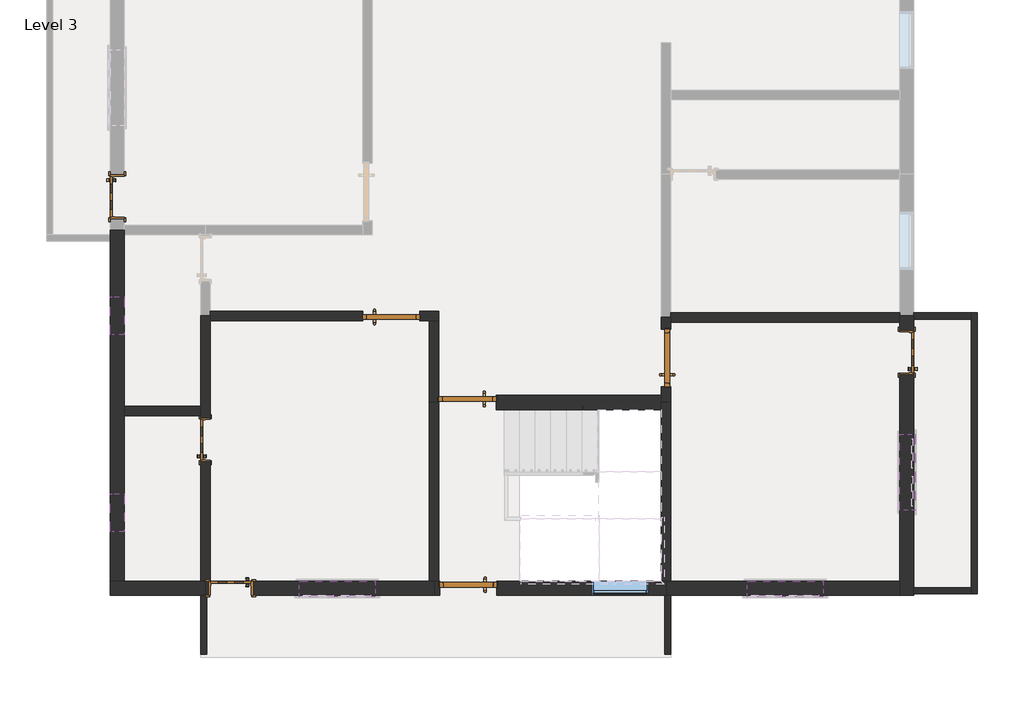
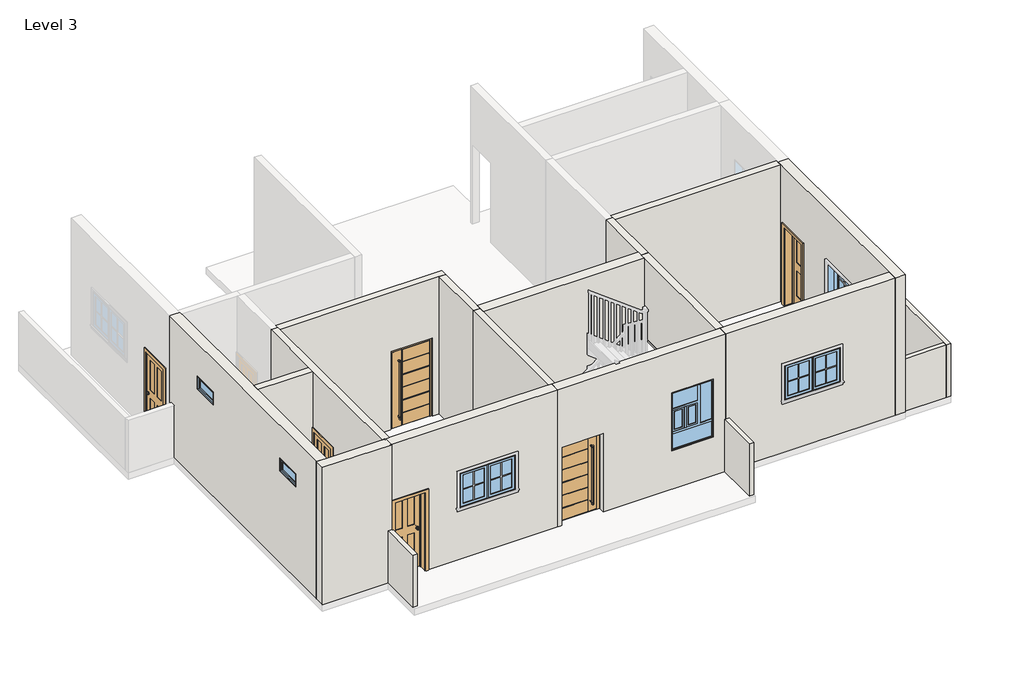
# One storey, part 1 of 3: 20 walls, 8 doors, 6 windows.
"""IFC4 building model written with IfcOpenShell, lengths in millimetres."""

from ifc_helpers import new_model, si_unit, frame, origin, place, context, project, spatial, polyline, outline, extrude, faceted_brep, transform, mapped, element, save
from components import door_3_44036f4b, door_3_3562bf2b, door_a03dd1d4, door_a34dad57, m_fixed_2_dd9f9b20, m_window_awning_double_horizontal_4_8afcb0b2, m_window_casement_double_sash_variable_3_661e274a

model = new_model("IFC4")

# Units and contexts
model_context = context("Model", 3, world=origin())
ifc_project = project(units=[si_unit("LENGTHUNIT", "METRE", prefix="MILLI")], contexts=[model_context])

# Site, building, storey
site = spatial("IfcSite", under=ifc_project)
building = spatial("IfcBuilding", under=site)
storey = spatial("IfcBuildingStorey", under=building, Name="Level 3", Elevation=6400.8)

# Doors
placement = place(None, origin())
door_3_shape = door_3_44036f4b(model_context)
element("IfcDoor", 1, ObjectType="3'", at=placement, inside=storey, context=model_context, shape_type="MappedRepresentation", body=[
    mapped(door_3_shape, transform((-13795.5794909, -9.3618509, 6400.8), x_axis=(1.0, 0.0, 0.0), y_axis=(0.0, 1.0, 0.0), z_axis=(0.0, 0.0, 1.0))),
])
element("IfcDoor", 2, ObjectType="3'", at=placement, inside=storey, context=model_context, shape_type="MappedRepresentation", body=[
    mapped(door_3_shape, transform((-9401.3794909, -682.4618509, 6400.8), x_axis=(0.0, 1.0, 0.0), y_axis=(-1.0, 0.0, 0.0), z_axis=(0.0, 0.0, 1.0))),
])
door_3_2_shape = door_3_3562bf2b(model_context)
element("IfcDoor", 3, ObjectType="3'", at=placement, inside=storey, context=model_context, shape_type="MappedRepresentation", body=[
    mapped(door_3_2_shape, transform((-12576.3794909, -1393.6618509, 6400.8), x_axis=(-1.0, 0.0, 0.0), y_axis=(0.0, -1.0, 0.0), z_axis=(0.0, 0.0, 1.0))),
])
element("IfcDoor", 4, ObjectType="3'", at=placement, inside=storey, context=model_context, shape_type="MappedRepresentation", body=[
    mapped(door_3_2_shape, transform((-12563.6794909, -4365.4618509, 6400.8), x_axis=(-1.0, 0.0, 0.0), y_axis=(0.0, -1.0, 0.0), z_axis=(0.0, 0.0, 1.0))),
])
door_shape = door_a03dd1d4(model_context)
element("IfcDoor", 5, ObjectType="M_Door-Interior-Single-4_Panel-Wood : 2'2\"", at=placement, inside=storey, context=model_context, shape_type="MappedRepresentation", body=[
    mapped(door_shape, transform((-16770.5544909, -1990.1618509, 6400.8), x_axis=(0.0, 1.0, 0.0), y_axis=(-1.0, 0.0, 0.0), z_axis=(0.0, 0.0, 1.0))),
])
door_2_shape = door_a34dad57(model_context)
element("IfcDoor", 6, ObjectType="M_Door-Interior-Single-4_Panel-Wood : 2'2\"", at=placement, inside=storey, context=model_context, shape_type="MappedRepresentation", body=[
    mapped(door_2_shape, transform((-18180.2544909, 1895.2381491, 6400.8), x_axis=(0.0, -1.0, 0.0), y_axis=(1.0, 0.0, 0.0), z_axis=(0.0, 0.0, 1.0))),
])
element("IfcDoor", 7, ObjectType="M_Door-Interior-Single-4_Panel-Wood : 2'2\"", at=placement, inside=storey, context=model_context, shape_type="MappedRepresentation", body=[
    mapped(door_2_shape, transform((-5550.1044909, -593.1618509, 6400.8), x_axis=(0.0, 1.0, 0.0), y_axis=(-1.0, 0.0, 0.0), z_axis=(0.0, 0.0, 1.0))),
])
element("IfcDoor", 8, ObjectType="M_Door-Interior-Single-4_Panel-Wood : 2'2\"", at=placement, inside=storey, context=model_context, shape_type="MappedRepresentation", body=[
    mapped(door_2_shape, transform((-16361.3794909, -4362.2868509, 6400.8), x_axis=(-1.0, 0.0, 0.0), y_axis=(0.0, -1.0, 0.0), z_axis=(0.0, 0.0, 1.0))),
])

# Walls
element("IfcWall", 9, ObjectType="Generic - 4\"", at=placement, inside=storey, context=model_context, shape_type="Brep", body=[
    faceted_brep([(-9325.1794909, -5419.5618509, 6400.8), (-9325.1794909, -4479.7618509, 6400.8), (-9325.1794909, -4479.7618509, 7620.0), (-9325.1794909, -5419.5618509, 7620.0), (-9426.7794909, -5419.5618509, 6400.8), (-9426.7794909, -5419.5618509, 7620.0), (-9426.7794909, -4479.7618509, 7620.0), (-9426.7794909, -4479.7618509, 6400.8), (-9401.3794909, -4479.7618509, 6400.8)], [[[0, 1, 2, 3]], [[4, 5, 6, 7]], [[1, 0, 4, 7, 8]], [[3, 2, 6, 5]], [[0, 3, 5, 4]], [[2, 1, 8, 7, 6]]]),
])
element("IfcWall", 10, ObjectType="Generic - 4\"", at=placement, inside=storey, context=model_context, shape_type="Brep", body=[
    faceted_brep([(-4422.9794909, -4454.3618509, 6400.8), (-4422.9794909, 41.4381491, 6400.8), (-4422.9794909, 41.4381491, 7620.0), (-4422.9794909, -4454.3618509, 7620.0), (-4524.5794909, -4454.3618509, 6400.8), (-4524.5794909, -4454.3618509, 7620.0), (-4524.5794909, -4352.7618509, 7620.0), (-4524.5794909, -60.1618509, 7620.0), (-4524.5794909, 41.4381491, 7620.0), (-4524.5794909, 41.4381491, 6400.8), (-4524.5794909, -60.1618509, 6400.8), (-4524.5794909, -4352.7618509, 6400.8)], [[[0, 1, 2, 3]], [[4, 5, 6, 7, 8, 9, 10, 11]], [[1, 0, 4, 11, 10, 9]], [[3, 2, 8, 7, 6, 5]], [[0, 3, 5, 4]], [[2, 1, 9, 8]]]),
])
element("IfcWall", 11, ObjectType="Generic - 4\"", at=placement, inside=storey, context=model_context, shape_type="SweptSolid", body=[
    extrude(outline(polyline([(-4524.5794909, -4454.3618509), (-5438.9794909, -4454.3618509), (-5438.9794909, -4352.7618509), (-4524.5794909, -4352.7618509), (-4524.5794909, -4454.3618509)])), frame((0.0, 0.0, 6400.8), z_axis=(0.0, 0.0, 1.0), x_axis=(1.0, 0.0, 0.0)), (0.0, 0.0, 1.0), 1219.2),
])
element("IfcWall", 12, ObjectType="Generic - 4\"", at=placement, inside=storey, context=model_context, shape_type="Brep", body=[
    faceted_brep([(-16843.5794909, -4479.7618509, 6400.8), (-16843.5794909, -5419.5618509, 6400.8), (-16843.5794909, -5419.5618509, 7620.0), (-16843.5794909, -4479.7618509, 7620.0), (-16741.9794909, -4479.7618509, 6400.8), (-16741.9794909, -4479.7618509, 7620.0), (-16741.9794909, -5419.5618509, 7620.0), (-16741.9794909, -5419.5618509, 6400.8), (-16792.7794909, -4479.7618509, 6400.8), (-16767.3794909, -4479.7618509, 6400.8)], [[[0, 1, 2, 3]], [[4, 5, 6, 7]], [[1, 0, 8, 9, 4, 7]], [[2, 1, 7, 6]], [[3, 2, 6, 5]], [[0, 3, 5, 4, 9, 8]]]),
])
element("IfcWall", 13, ObjectType="Generic - 4\"", at=placement, inside=storey, context=model_context, shape_type="Brep", body=[
    faceted_brep([(-4524.5794909, 41.4381491, 6400.8), (-5438.9794909, 41.4381491, 6400.8), (-5438.9794909, 41.4381491, 7620.0), (-4524.5794909, 41.4381491, 7620.0), (-4524.5794909, -60.1618509, 6400.8), (-4524.5794909, -60.1618509, 7620.0), (-5438.9794909, -60.1618509, 7620.0), (-5438.9794909, -60.1618509, 6400.8), (-5438.9794909, -34.7618509, 6400.8), (-5438.9794909, -9.3618509, 6400.8)], [[[0, 1, 2, 3]], [[4, 5, 6, 7]], [[1, 0, 4, 7, 8, 9]], [[3, 2, 6, 5]], [[0, 3, 5, 4]], [[2, 1, 9, 8, 7, 6]]]),
])
element("IfcWall", 14, ObjectType="Generic - 6\"", at=placement, inside=storey, context=model_context, shape_type="Brep", body=[
    faceted_brep([(-16691.1794909, -9.3618509, 6400.8), (-16691.1794909, -9.3618509, 9601.2), (-16691.1794909, -85.5618509, 9601.2), (-16691.1794909, -4251.1618509, 9601.2), (-16691.1794909, -4251.1618509, 6400.8), (-16691.1794909, -2345.3618509, 6400.8), (-16691.1794909, -2345.3618509, 8254.6), (-16691.1794909, -1634.9618509, 8254.6), (-16691.1794909, -1634.9618509, 6400.8), (-16691.1794909, -85.5618509, 6400.8), (-16843.5794909, -9.3618509, 9601.2), (-16843.5794909, -9.3618509, 6400.8), (-16843.5794909, -1457.1618509, 6400.8), (-16843.5794909, -1609.5618509, 6400.8), (-16843.5794909, -1634.9618509, 6400.8), (-16843.5794909, -1634.9618509, 8254.6), (-16843.5794909, -2345.3618509, 8254.6), (-16843.5794909, -2345.3618509, 6400.8), (-16843.5794909, -4251.1618509, 6400.8), (-16843.5794909, -4251.1618509, 9601.2), (-16843.5794909, -1609.5618509, 9601.2), (-16843.5794909, -1457.1618509, 9601.2), (-16716.5794909, -4251.1618509, 6400.8), (-16767.3794909, -4251.1618509, 6400.8), (-16792.7794909, -4251.1618509, 6400.8), (-16792.7794909, -4251.1618509, 9601.2), (-16767.3794909, -4251.1618509, 9601.2)], [[[0, 1, 2, 3, 4, 5, 6, 7, 8, 9]], [[10, 11, 12, 13, 14, 15, 16, 17, 18, 19, 20, 21]], [[4, 22, 23, 24, 18, 17, 5]], [[11, 0, 9, 8, 14, 13, 12]], [[1, 0, 11, 10]], [[3, 2, 1, 10, 21, 20, 19, 25, 26]], [[7, 15, 14, 8]], [[15, 7, 6, 16]], [[16, 6, 5, 17]], [[3, 26, 25, 19, 18, 24, 23, 22, 4]]]),
])
element("IfcWall", 15, ObjectType="Generic - 6\"", at=placement, inside=storey, context=model_context, shape_type="SweptSolid", body=[
    extrude(outline(polyline([(-16843.5794909, -1609.5618509), (-18062.7794909, -1609.5618509), (-18062.7794909, -1457.1618509), (-16843.5794909, -1457.1618509), (-16843.5794909, -1609.5618509)])), frame((0.0, 0.0, 6400.8), z_axis=(0.0, 0.0, 1.0), x_axis=(1.0, 0.0, 0.0)), (0.0, 0.0, 1.0), 3200.4),
])
element("IfcWall", 16, ObjectType="Generic - 6\"", at=placement, inside=storey, context=model_context, shape_type="Brep", body=[
    faceted_brep([(-13033.5794909, -85.5618509, 9601.2), (-13185.9794909, -85.5618509, 9601.2), (-16691.1794909, -85.5618509, 9601.2), (-16691.1794909, -85.5618509, 6400.8), (-14252.7794909, -85.5618509, 6400.8), (-14252.7794909, -85.5618509, 8229.6), (-13338.3794909, -85.5618509, 8229.6), (-13338.3794909, -85.5618509, 6400.8), (-13185.9794909, -85.5618509, 6400.8), (-13033.5794909, -85.5618509, 6400.8), (-16691.1794909, 66.8381491, 9601.2), (-13033.5794909, 66.8381491, 9601.2), (-13033.5794909, 66.8381491, 6400.8), (-13338.3794909, 66.8381491, 6400.8), (-13338.3794909, 66.8381491, 8229.6), (-14252.7794909, 66.8381491, 8229.6), (-14252.7794909, 66.8381491, 6400.8), (-16691.1794909, 66.8381491, 6400.8), (-13338.3794909, -65.5618509, 6400.8), (-13323.3794909, -65.5618509, 6400.8), (-13323.3794909, 11.4381491, 6400.8), (-13338.3794909, 11.4381491, 6400.8), (-16691.1794909, -9.3618509, 6400.8), (-14252.7794909, 11.4381491, 6400.8), (-14267.7794909, 11.4381491, 6400.8), (-14267.7794909, -65.5618509, 6400.8), (-14252.7794909, -65.5618509, 6400.8), (-16691.1794909, -9.3618509, 9601.2), (-14252.7794909, -65.5618509, 8229.6), (-13338.3794909, -65.5618509, 8229.6), (-13338.3794909, 11.4381491, 8229.6), (-14252.7794909, 11.4381491, 8229.6), (-14267.7794909, -65.5618509, 8244.6), (-14267.7794909, 11.4381491, 8244.6), (-13323.3794909, 11.4381491, 8244.6), (-13323.3794909, -65.5618509, 8244.6)], [[[0, 1, 2, 3, 4, 5, 6, 7, 8, 9]], [[10, 11, 12, 13, 14, 15, 16, 17]], [[12, 9, 8, 7, 18, 19, 20, 21, 13]], [[3, 22, 17, 16, 23, 24, 25, 26, 4]], [[2, 1, 0, 11, 10, 27]], [[3, 2, 27, 10, 17, 22]], [[0, 9, 12, 11]], [[5, 28, 29, 6]], [[14, 30, 31, 15]], [[6, 29, 18, 7]], [[30, 14, 13, 21]], [[28, 5, 4, 26]], [[15, 31, 23, 16]], [[32, 33, 34, 35]], [[35, 34, 20, 19]], [[31, 30, 21, 20, 34, 33, 24, 23]], [[33, 32, 25, 24]], [[29, 28, 26, 25, 32, 35, 19, 18]]]),
])
element("IfcWall", 17, ObjectType="Generic - 6\"", at=placement, inside=storey, context=model_context, shape_type="Brep", body=[
    faceted_brep([(-13185.9794909, -85.5618509, 6400.8), (-13185.9794909, -1393.6618509, 6400.8), (-13185.9794909, -1393.6618509, 9601.2), (-13185.9794909, -85.5618509, 9601.2), (-13033.5794909, -85.5618509, 9601.2), (-13033.5794909, -1279.3618509, 9601.2), (-13033.5794909, -1393.6618509, 9601.2), (-13033.5794909, -1393.6618509, 8229.6), (-13033.5794909, -1393.6618509, 6400.8), (-13033.5794909, -1376.3618508, 6400.8), (-13033.5794909, -1376.3618508, 8229.6), (-13033.5794909, -1376.3618508, 8244.6), (-13033.5794909, -1299.3618508, 8244.6), (-13033.5794909, -1299.3618508, 8229.6), (-13033.5794909, -1299.3618508, 6400.8), (-13033.5794909, -1279.3618508, 6400.8), (-13033.5794909, -85.5618509, 6400.8), (-13048.5794909, -1299.3618508, 6400.8), (-13048.5794909, -1376.3618508, 6400.8), (-13048.5794909, -1376.3618508, 8244.6), (-13048.5794909, -1299.3618508, 8244.6)], [[[0, 1, 2, 3]], [[4, 5, 6, 7, 8, 9, 10, 11, 12, 13, 14, 15, 16]], [[1, 0, 16, 15, 14, 17, 18, 9, 8]], [[2, 1, 8, 7, 6]], [[3, 2, 6, 5, 4]], [[0, 3, 4, 16]], [[19, 20, 12, 11]], [[20, 19, 18, 17]], [[18, 19, 11, 10, 9]], [[20, 17, 14, 13, 12]]]),
])
element("IfcWall", 18, ObjectType="Generic - 6\"", at=placement, inside=storey, context=model_context, shape_type="Brep", body=[
    faceted_brep([(-9325.1794909, -4251.1618509, 9601.2), (-9325.1794909, -4251.1618509, 6400.8), (-9325.1794909, -1393.6618509, 6400.8), (-9325.1794909, -1393.6618509, 9601.2), (-9477.5794909, -4251.1618509, 6400.8), (-9477.5794909, -4251.1618509, 9601.2), (-9477.5794909, -1507.9618509, 9601.2), (-9477.5794909, -1393.6618509, 9601.2), (-9477.5794909, -1393.6618509, 6400.8), (-9477.5794909, -1507.9618509, 6400.8), (-9401.3794909, -4251.1618509, 6400.8), (-9401.3794909, -4251.1618509, 9601.2)], [[[0, 1, 2, 3]], [[4, 5, 6, 7, 8, 9]], [[2, 1, 10, 4, 9, 8]], [[3, 2, 8, 7]], [[0, 3, 7, 6, 5, 11]], [[0, 11, 5, 4, 10, 1]]]),
])
element("IfcWall", 19, ObjectType="Generic - 6\"", at=placement, inside=storey, context=model_context, shape_type="Brep", body=[
    faceted_brep([(-5667.5794909, 41.4381491, 9601.2), (-5667.5794909, 41.4381491, 6400.8), (-9325.1794909, 41.4381491, 6400.8), (-9325.1794909, 41.4381491, 9601.2), (-5667.5794909, -110.9618509, 6400.8), (-5667.5794909, -110.9618509, 9601.2), (-9325.1794909, -110.9618509, 9601.2), (-9325.1794909, -110.9618509, 6400.8), (-5667.5794909, -9.3618509, 6400.8), (-5667.5794909, -34.7618509, 6400.8), (-9325.1794909, -34.7618509, 6400.8), (-9325.1794909, -34.7618509, 9601.2), (-5667.5794909, -34.7618509, 9601.2), (-5667.5794909, -9.3618509, 9601.2)], [[[0, 1, 2, 3]], [[4, 5, 6, 7]], [[2, 1, 8, 9, 4, 7, 10]], [[0, 3, 11, 6, 5, 12, 13]], [[3, 2, 10, 7, 6, 11]], [[0, 13, 12, 5, 4, 9, 8, 1]]]),
])
element("IfcWall", 20, ObjectType="Generic - 6\"", at=placement, inside=storey, context=model_context, shape_type="Brep", body=[
    faceted_brep([(-9325.1794909, -34.7618509, 6400.8), (-9325.1794909, -34.7618509, 9601.2), (-9325.1794909, -110.9618509, 9601.2), (-9325.1794909, -1393.6618509, 9601.2), (-9325.1794909, -1393.6618509, 6400.8), (-9325.1794909, -1139.6618509, 6400.8), (-9325.1794909, -1139.6618509, 8229.6), (-9325.1794909, -225.2618509, 8229.6), (-9325.1794909, -225.2618509, 6400.8), (-9325.1794909, -110.9618509, 6400.8), (-9477.5794909, -34.7618509, 9601.2), (-9477.5794909, -34.7618509, 6400.8), (-9477.5794909, -225.2618509, 6400.8), (-9477.5794909, -225.2618509, 8229.6), (-9477.5794909, -1139.6618509, 8229.6), (-9477.5794909, -1139.6618509, 6400.8), (-9477.5794909, -1279.3618509, 6400.8), (-9477.5794909, -1393.6618509, 6400.8), (-9477.5794909, -1393.6618509, 9601.2), (-9477.5794909, -1279.3618509, 9601.2), (-9345.1794909, -225.2618509, 6400.8), (-9345.1794909, -210.2618509, 6400.8), (-9422.1794909, -210.2618509, 6400.8), (-9422.1794909, -225.2618509, 6400.8), (-9422.1794909, -1139.6618509, 6400.8), (-9422.1794909, -1154.6618509, 6400.8), (-9345.1794909, -1154.6618509, 6400.8), (-9345.1794909, -1139.6618509, 6400.8), (-9345.1794909, -1139.6618509, 8229.6), (-9345.1794909, -225.2618509, 8229.6), (-9422.1794909, -225.2618509, 8229.6), (-9422.1794909, -1139.6618509, 8229.6), (-9345.1794909, -1154.6618509, 8244.6), (-9422.1794909, -1154.6618509, 8244.6), (-9422.1794909, -210.2618509, 8244.6), (-9345.1794909, -210.2618509, 8244.6)], [[[0, 1, 2, 3, 4, 5, 6, 7, 8, 9]], [[10, 11, 12, 13, 14, 15, 16, 17, 18, 19]], [[11, 0, 9, 8, 20, 21, 22, 23, 12]], [[4, 17, 16, 15, 24, 25, 26, 27, 5]], [[1, 0, 11, 10]], [[3, 2, 1, 10, 19, 18]], [[4, 3, 18, 17]], [[6, 28, 29, 7]], [[13, 30, 31, 14]], [[30, 13, 12, 23]], [[7, 29, 20, 8]], [[14, 31, 24, 15]], [[28, 6, 5, 27]], [[32, 33, 34, 35]], [[35, 34, 22, 21]], [[31, 30, 23, 22, 34, 33, 25, 24]], [[33, 32, 26, 25]], [[29, 28, 27, 26, 32, 35, 21, 20]]]),
])
element("IfcWall", 21, ObjectType="Generic - 6\"", at=placement, inside=storey, context=model_context, shape_type="Brep", body=[
    faceted_brep([(-13185.9794909, -1393.6618509, 6400.8), (-13185.9794909, -4251.1618509, 6400.8), (-13185.9794909, -4251.1618509, 9601.2), (-13185.9794909, -1393.6618509, 9601.2), (-13033.5794909, -1393.6618509, 9601.2), (-13033.5794909, -1507.9618509, 9601.2), (-13033.5794909, -4251.1618509, 9601.2), (-13033.5794909, -4251.1618509, 6400.8), (-13033.5794909, -1507.9618509, 6400.8), (-13033.5794909, -1393.6618509, 6400.8), (-13033.5794909, -1393.6618509, 8229.6), (-13109.7794909, -4251.1618509, 6400.8), (-13109.7794909, -4251.1618509, 9601.2)], [[[0, 1, 2, 3]], [[4, 5, 6, 7, 8, 9, 10]], [[1, 0, 9, 8, 7, 11]], [[3, 2, 12, 6, 5, 4]], [[0, 3, 4, 10, 9]], [[2, 1, 11, 7, 6, 12]]]),
])
element("IfcWall", 22, ObjectType="Generic - 9\"", at=placement, inside=storey, context=model_context, shape_type="Brep", body=[
    faceted_brep([(-5667.5794909, -4251.1618509, 9601.2), (-5667.5794909, -4251.1618509, 6400.8), (-9325.1794909, -4251.1618509, 6400.8), (-9401.3794909, -4251.1618509, 6400.8), (-9401.3794909, -4251.1618509, 9601.2), (-9325.1794909, -4251.1618509, 9601.2), (-8105.9794909, -4251.1618509, 8420.0), (-8105.9794909, -4251.1618509, 7620.0), (-6886.7794909, -4251.1618509, 7620.0), (-6886.7794909, -4251.1618509, 8420.0), (-5667.5794909, -4479.7618509, 6400.8), (-5667.5794909, -4479.7618509, 9601.2), (-9401.3794909, -4479.7618509, 9601.2), (-9401.3794909, -4479.7618509, 6400.8), (-9325.1794909, -4479.7618509, 6400.8), (-8105.9794909, -4479.7618509, 8420.0), (-6886.7794909, -4479.7618509, 8420.0), (-6886.7794909, -4479.7618509, 7620.0), (-8105.9794909, -4479.7618509, 7620.0)], [[[0, 1, 2, 3, 4, 5], [6, 7, 8, 9]], [[10, 11, 12, 13, 14], [15, 16, 17, 18]], [[3, 2, 1, 10, 14, 13]], [[4, 3, 13, 12]], [[0, 5, 4, 12, 11]], [[0, 11, 10, 1]], [[7, 6, 15, 18]], [[8, 7, 18, 17]], [[9, 8, 17, 16]], [[6, 9, 16, 15]]]),
])
element("IfcWall", 23, ObjectType="Generic - 9\"", at=placement, inside=storey, context=model_context, shape_type="Brep", body=[
    faceted_brep([(-18062.7794909, -4251.1618509, 6400.8), (-18062.7794909, -1609.5618509, 6400.8), (-18062.7794909, -1457.1618509, 6400.8), (-18062.7794909, 1286.0381491, 6400.8), (-18062.7794909, 1362.2381491, 6400.8), (-18062.7794909, 1362.2381491, 9601.2), (-18062.7794909, 1286.0381491, 9601.2), (-18062.7794909, -1457.1618509, 9601.2), (-18062.7794909, -1609.5618509, 9601.2), (-18062.7794909, -4251.1618509, 9601.2), (-18062.7794909, -3463.7618509, 8534.4), (-18062.7794909, -3463.7618509, 8839.2), (-18062.7794909, -2854.1618509, 8839.2), (-18062.7794909, -2854.1618509, 8534.4), (-18062.7794909, -314.1618509, 8534.4), (-18062.7794909, -314.1618509, 8839.2), (-18062.7794909, 295.4381491, 8839.2), (-18062.7794909, 295.4381491, 8534.4), (-18291.3794909, -4251.1618509, 6400.8), (-18291.3794909, -4251.1618509, 9601.2), (-18291.3794909, 1362.2381491, 9601.2), (-18291.3794909, 1362.2381491, 6400.8), (-18291.3794909, 1286.0381491, 6400.8), (-18291.3794909, 1184.4381491, 6400.8), (-18291.3794909, -3463.7618509, 8534.4), (-18291.3794909, -2854.1618509, 8534.4), (-18291.3794909, -2854.1618509, 8839.2), (-18291.3794909, -3463.7618509, 8839.2), (-18291.3794909, -314.1618509, 8534.4), (-18291.3794909, 295.4381491, 8534.4), (-18291.3794909, 295.4381491, 8839.2), (-18291.3794909, -314.1618509, 8839.2)], [[[0, 1, 2, 3, 4, 5, 6, 7, 8, 9], [10, 11, 12, 13], [14, 15, 16, 17]], [[18, 19, 20, 21, 22, 23], [24, 25, 26, 27], [28, 29, 30, 31]], [[4, 3, 2, 1, 0, 18, 23, 22, 21]], [[9, 8, 7, 6, 5, 20, 19]], [[0, 9, 19, 18]], [[11, 10, 24, 27]], [[12, 11, 27, 26]], [[13, 12, 26, 25]], [[10, 13, 25, 24]], [[15, 14, 28, 31]], [[16, 15, 31, 30]], [[17, 16, 30, 29]], [[14, 17, 29, 28]], [[4, 21, 20, 5]]]),
])
element("IfcWall", 24, ObjectType="Generic - 9\"", at=placement, inside=storey, context=model_context, shape_type="Brep", body=[
    faceted_brep([(-13033.5794909, -1279.3618509, 9601.2), (-9477.5794909, -1279.3618509, 9601.2), (-9477.5794909, -1279.3618509, 6400.8), (-12119.1794909, -1279.3618509, 6400.8), (-12119.1794909, -1279.3618509, 8229.6), (-13033.5794909, -1279.3618509, 8229.6), (-9477.5794909, -1507.9618509, 9601.2), (-13033.5794909, -1507.9618509, 9601.2), (-13033.5794909, -1507.9618509, 8229.6), (-12119.1794909, -1507.9618509, 8229.6), (-12119.1794909, -1507.9618509, 6400.8), (-9477.5794909, -1507.9618509, 6400.8), (-9477.5794909, -1393.6618509, 6400.8), (-12119.1794909, -1376.3618508, 6400.8), (-12104.1794909, -1376.3618508, 6400.8), (-12104.1794909, -1299.3618508, 6400.8), (-12119.1794909, -1299.3618508, 6400.8), (-13033.5794909, -1393.6618509, 9601.2), (-9477.5794909, -1393.6618509, 9601.2), (-13033.5794909, -1299.3618508, 8229.6), (-13033.5794909, -1299.3618508, 8244.6), (-13033.5794909, -1376.3618508, 8244.6), (-13033.5794909, -1376.3618508, 8229.6), (-12119.1794909, -1299.3618508, 8229.6), (-12119.1794909, -1376.3618508, 8229.6), (-12104.1794909, -1299.3618508, 8244.6), (-12104.1794909, -1376.3618508, 8244.6)], [[[0, 1, 2, 3, 4, 5]], [[6, 7, 8, 9, 10, 11]], [[2, 12, 11, 10, 13, 14, 15, 16, 3]], [[1, 0, 17, 7, 6, 18]], [[7, 17, 0, 5, 19, 20, 21, 22, 8]], [[2, 1, 18, 6, 11, 12]], [[4, 23, 19, 5]], [[22, 24, 9, 8]], [[23, 4, 3, 16]], [[9, 24, 13, 10]], [[25, 26, 21, 20]], [[24, 22, 21, 26, 14, 13]], [[26, 25, 15, 14]], [[19, 23, 16, 15, 25, 20]]]),
])
element("IfcWall", 25, ObjectType="Generic - 9\"", at=placement, inside=storey, context=model_context, shape_type="Brep", body=[
    faceted_brep([(-5667.5794909, -4479.7618509, 9601.2), (-5667.5794909, -4251.1618509, 9601.2), (-5667.5794909, -110.9618509, 9601.2), (-5667.5794909, -9.3618509, 9601.2), (-5667.5794909, -9.3618509, 6400.8), (-5667.5794909, -110.9618509, 6400.8), (-5667.5794909, -237.9618509, 6400.8), (-5667.5794909, -237.9618509, 8254.6), (-5667.5794909, -948.3618509, 8254.6), (-5667.5794909, -948.3618509, 6400.8), (-5667.5794909, -4251.1618509, 6400.8), (-5667.5794909, -4479.7618509, 6400.8), (-5667.5794909, -3120.0618509, 8420.0), (-5667.5794909, -3120.0618509, 7620.0), (-5667.5794909, -1900.8618509, 7620.0), (-5667.5794909, -1900.8618509, 8420.0), (-5438.9794909, -9.3618509, 9601.2), (-5438.9794909, -4479.7618509, 9601.2), (-5438.9794909, -4479.7618509, 6400.8), (-5438.9794909, -4454.3618509, 6400.8), (-5438.9794909, -4352.7618509, 6400.8), (-5438.9794909, -948.3618509, 6400.8), (-5438.9794909, -948.3618509, 8254.6), (-5438.9794909, -237.9618509, 8254.6), (-5438.9794909, -237.9618509, 6400.8), (-5438.9794909, -60.1618509, 6400.8), (-5438.9794909, -9.3618509, 6400.8), (-5438.9794909, -3120.0618509, 8420.0), (-5438.9794909, -1900.8618509, 8420.0), (-5438.9794909, -1900.8618509, 7620.0), (-5438.9794909, -3120.0618509, 7620.0)], [[[0, 1, 2, 3, 4, 5, 6, 7, 8, 9, 10, 11], [12, 13, 14, 15]], [[16, 17, 18, 19, 20, 21, 22, 23, 24, 25, 26], [27, 28, 29, 30]], [[4, 26, 25, 24, 6, 5]], [[18, 11, 10, 9, 21, 20, 19]], [[3, 2, 1, 0, 17, 16]], [[11, 18, 17, 0]], [[12, 15, 28, 27]], [[15, 14, 29, 28]], [[14, 13, 30, 29]], [[13, 12, 27, 30]], [[3, 16, 26, 4]], [[23, 7, 6, 24]], [[7, 23, 22, 8]], [[8, 22, 21, 9]]]),
])
element("IfcWall", 26, ObjectType="Generic - 9\"", at=placement, inside=storey, context=model_context, shape_type="Brep", body=[
    faceted_brep([(-13109.7794909, -4251.1618509, 6400.8), (-13109.7794909, -4251.1618509, 9601.2), (-13033.5794909, -4251.1618509, 9601.2), (-9477.5794909, -4251.1618509, 9601.2), (-9401.3794909, -4251.1618509, 9601.2), (-9401.3794909, -4251.1618509, 6400.8), (-9477.5794909, -4251.1618509, 6400.8), (-12106.4794909, -4251.1618509, 6400.8), (-12106.4794909, -4251.1618509, 8229.6), (-13020.8794909, -4251.1618509, 8229.6), (-13020.8794909, -4251.1618509, 6400.8), (-13033.5794909, -4251.1618509, 6400.8), (-10595.1794909, -4251.1618509, 8650.8), (-10595.1794909, -4251.1618509, 7300.8), (-9680.7794909, -4251.1618509, 7300.8), (-9680.7794909, -4251.1618509, 8650.8), (-13109.7794909, -4479.7618509, 9601.2), (-13109.7794909, -4479.7618509, 6400.8), (-13020.8794909, -4479.7618509, 6400.8), (-13020.8794909, -4479.7618509, 8229.6), (-12106.4794909, -4479.7618509, 8229.6), (-12106.4794909, -4479.7618509, 6400.8), (-9426.7794909, -4479.7618509, 6400.8), (-9401.3794909, -4479.7618509, 6400.8), (-9401.3794909, -4479.7618509, 9601.2), (-10595.1794909, -4479.7618509, 8650.8), (-9680.7794909, -4479.7618509, 8650.8), (-9680.7794909, -4479.7618509, 7300.8), (-10595.1794909, -4479.7618509, 7300.8), (-12106.4794909, -4348.1618508, 6400.8), (-12091.4794909, -4348.1618508, 6400.8), (-12091.4794909, -4271.1618508, 6400.8), (-12106.4794909, -4271.1618508, 6400.8), (-13020.8794909, -4271.1618508, 6400.8), (-13035.8794909, -4271.1618508, 6400.8), (-13035.8794909, -4348.1618508, 6400.8), (-13020.8794909, -4348.1618508, 6400.8), (-12106.4794909, -4271.1618508, 8229.6), (-13020.8794909, -4271.1618508, 8229.6), (-13020.8794909, -4348.1618508, 8229.6), (-12106.4794909, -4348.1618508, 8229.6), (-12091.4794909, -4271.1618508, 8244.6), (-12091.4794909, -4348.1618508, 8244.6), (-13035.8794909, -4348.1618508, 8244.6), (-13035.8794909, -4271.1618508, 8244.6)], [[[0, 1, 2, 3, 4, 5, 6, 7, 8, 9, 10, 11], [12, 13, 14, 15]], [[16, 17, 18, 19, 20, 21, 22, 23, 24], [25, 26, 27, 28]], [[5, 23, 22, 21, 29, 30, 31, 32, 7, 6]], [[17, 0, 11, 10, 33, 34, 35, 36, 18]], [[1, 0, 17, 16]], [[4, 3, 2, 1, 16, 24]], [[8, 37, 38, 9]], [[19, 39, 40, 20]], [[39, 19, 18, 36]], [[9, 38, 33, 10]], [[20, 40, 29, 21]], [[37, 8, 7, 32]], [[41, 42, 43, 44]], [[44, 43, 35, 34]], [[40, 39, 36, 35, 43, 42, 30, 29]], [[42, 41, 31, 30]], [[38, 37, 32, 31, 41, 44, 34, 33]], [[12, 15, 26, 25]], [[15, 14, 27, 26]], [[14, 13, 28, 27]], [[13, 12, 25, 28]], [[4, 24, 23, 5]]]),
])
element("IfcWall", 27, ObjectType="Generic - 9\"", at=placement, inside=storey, context=model_context, shape_type="Brep", body=[
    faceted_brep([(-16792.7794909, -4251.1618509, 9601.2), (-16691.1794909, -4251.1618509, 9601.2), (-13185.9794909, -4251.1618509, 9601.2), (-13109.7794909, -4251.1618509, 9601.2), (-13109.7794909, -4251.1618509, 6400.8), (-13185.9794909, -4251.1618509, 6400.8), (-16006.1794909, -4251.1618509, 6400.8), (-16006.1794909, -4251.1618509, 8254.6), (-16716.5794909, -4251.1618509, 8254.6), (-16716.5794909, -4251.1618509, 6400.8), (-16792.7794909, -4251.1618509, 6400.8), (-15269.5794909, -4251.1618509, 8420.0), (-15269.5794909, -4251.1618509, 7620.0), (-14050.3794909, -4251.1618509, 7620.0), (-14050.3794909, -4251.1618509, 8420.0), (-13109.7794909, -4479.7618509, 9601.2), (-16792.7794909, -4479.7618509, 9601.2), (-16792.7794909, -4479.7618509, 6400.8), (-16741.9794909, -4479.7618509, 6400.8), (-16716.5794909, -4479.7618509, 6400.8), (-16716.5794909, -4479.7618509, 8254.6), (-16006.1794909, -4479.7618509, 8254.6), (-16006.1794909, -4479.7618509, 6400.8), (-13109.7794909, -4479.7618509, 6400.8), (-15269.5794909, -4479.7618509, 8420.0), (-14050.3794909, -4479.7618509, 8420.0), (-14050.3794909, -4479.7618509, 7620.0), (-15269.5794909, -4479.7618509, 7620.0)], [[[0, 1, 2, 3, 4, 5, 6, 7, 8, 9, 10], [11, 12, 13, 14]], [[15, 16, 17, 18, 19, 20, 21, 22, 23], [24, 25, 26, 27]], [[17, 10, 9, 19, 18]], [[4, 23, 22, 6, 5]], [[3, 2, 1, 0, 16, 15]], [[4, 3, 15, 23]], [[11, 14, 25, 24]], [[14, 13, 26, 25]], [[13, 12, 27, 26]], [[12, 11, 24, 27]], [[8, 20, 19, 9]], [[20, 8, 7, 21]], [[21, 7, 6, 22]], [[10, 17, 16, 0]]]),
])
element("IfcWall", 28, ObjectType="Generic - 9\"", at=placement, inside=storey, context=model_context, shape_type="Brep", body=[
    faceted_brep([(-16767.3794909, -4251.1618509, 9601.2), (-16767.3794909, -4251.1618509, 6400.8), (-16843.5794909, -4251.1618509, 6400.8), (-18062.7794909, -4251.1618509, 6400.8), (-18291.3794909, -4251.1618509, 6400.8), (-18291.3794909, -4251.1618509, 9601.2), (-18062.7794909, -4251.1618509, 9601.2), (-16843.5794909, -4251.1618509, 9601.2), (-16767.3794909, -4479.7618509, 6400.8), (-16767.3794909, -4479.7618509, 9601.2), (-18291.3794909, -4479.7618509, 9601.2), (-18291.3794909, -4479.7618509, 6400.8), (-16843.5794909, -4479.7618509, 6400.8)], [[[0, 1, 2, 3, 4, 5, 6, 7]], [[8, 9, 10, 11, 12]], [[4, 3, 2, 1, 8, 12, 11]], [[0, 7, 6, 5, 10, 9]], [[5, 4, 11, 10]], [[0, 9, 8, 1]]]),
])

# Windows
m_fixed_2_shape = m_fixed_2_dd9f9b20(model_context)
element("IfcWindow", 29, ObjectType="M_Fixed : 2'", at=placement, inside=storey, context=model_context, shape_type="MappedRepresentation", body=[
    mapped(m_fixed_2_shape, transform((-18164.0794909, -3158.9618509, 7619.4), x_axis=(0.0, 1.0, 0.0), y_axis=(-1.0, 0.0, 0.0), z_axis=(0.0, 0.0, 1.0))),
])
element("IfcWindow", 30, ObjectType="M_Fixed : 2'", at=placement, inside=storey, context=model_context, shape_type="MappedRepresentation", body=[
    mapped(m_fixed_2_shape, transform((-18164.0794909, -9.3618509, 7619.4), x_axis=(0.0, 1.0, 0.0), y_axis=(-1.0, 0.0, 0.0), z_axis=(0.0, 0.0, 1.0))),
])
m_window_awning_double_horizontal_4_shape = m_window_awning_double_horizontal_4_8afcb0b2(model_context)
element("IfcWindow", 31, ObjectType="M_Window-Awning-Double-Horizontal : 4'", at=placement, inside=storey, context=model_context, shape_type="MappedRepresentation", body=[
    mapped(m_window_awning_double_horizontal_4_shape, transform((-14659.9794909, -4365.4618509, 6720.0), x_axis=(-1.0, 0.0, 0.0), y_axis=(0.0, -1.0, 0.0), z_axis=(0.0, 0.0, 1.0))),
])
element("IfcWindow", 32, ObjectType="M_Window-Awning-Double-Horizontal : 4'", at=placement, inside=storey, context=model_context, shape_type="MappedRepresentation", body=[
    mapped(m_window_awning_double_horizontal_4_shape, transform((-5553.2794909, -2510.4618509, 6720.0), x_axis=(0.0, -1.0, 0.0), y_axis=(1.0, 0.0, 0.0), z_axis=(0.0, 0.0, 1.0))),
])
element("IfcWindow", 33, ObjectType="M_Window-Awning-Double-Horizontal : 4'", at=placement, inside=storey, context=model_context, shape_type="MappedRepresentation", body=[
    mapped(m_window_awning_double_horizontal_4_shape, transform((-7496.3794909, -4365.4618509, 6720.0), x_axis=(-1.0, 0.0, 0.0), y_axis=(0.0, -1.0, 0.0), z_axis=(0.0, 0.0, 1.0))),
])
m_window_casement_double_sash_variable_3_shape = m_window_casement_double_sash_variable_3_661e274a(model_context)
element("IfcWindow", 34, ObjectType="M_Window-Casement-Double-Sash-Variable : 3'", at=placement, inside=storey, context=model_context, shape_type="MappedRepresentation", body=[
    mapped(m_window_casement_double_sash_variable_3_shape, transform((-10137.9794909, -4365.4618509, 6400.8), x_axis=(-1.0, 0.0, 0.0), y_axis=(0.0, -1.0, 0.0), z_axis=(0.0, 0.0, 1.0))),
])

save(model, "model.ifc")

# Revit data of these elements
# Type "3'"
#   Type Mark = "41"
#   Water resistance = "up to Class E900, EN 12208:2001"
#   Uniclass2015Version = "v1.21"
#   Uniclass2015Reference = "Ss_25_30_20_30"
#   Uniclass2015Description = "Frame and door leaf system"
#   URL = "www.aluprof.com"
#   Type IFC Predefined Type = "USERDEFINED"
#   Right-hand / Left-hand door [instance default] = ""
#   Resistance to wind load = "up to Class C5/B5, EN 12210:2001"
#   Insert type = "ST"
#   Hardware [instance default] = ""
#   Product page = "https://aluprof.com/en/architects/offer/window-and-door-systems/panel-doors#visualisation"
#   Operation = "SinglePanelOutwardOpening"
#   Opening type = "Outward"
#   NBSReference = "25-50-20/125"
#   NBSDescription = "Frame and door leaf system"
#   Important = "The actual acceptable construction dimensions are dependent on the selection of profiles and hardware, glazing type, construction weight and the construction’s operating conditions. These should be determined by a suitably qualified person, and using ALUPROF’s calculation software"
#   IfcExportType = "USERDEFINED"
#   IfcExportAs = "IfcDoorType"
#   Handle type [instance default] = ""
#   Manufacturer = "ALUPROF SA"
#   Export Type to IFC As = "IfcDoorType"
#   Door sill type [instance default] = ""
#   Description = "External single-leaf panel door outward opening"
#   Model = "MB-86 ST Panel Door AD07"
#   Content of the recyclate in the material = "69.2%"
#   COBie.Type.WarrantyDurationParts = ""
#   COBie.Type.Name = ""
#   COBie.Type.Manufacturer = "ALUPROF SA"
#   COBie.Space.Name = ""
#   COBie.Floor.Name = ""
#   COBie.Facility.Name = ""
#   COBie.CreatedOn = ""
#   COBie.Component.WarrantyStartDate = ""
#   COBie.Component.Name = "MB-86 ST Panel Door AD07"
#   Burglar resistance = "RC2"
#   Air permeability = "up to Class 4, EN 12207:2001"
#   Width of the active leaf = 2' - 8.17717"
#   Placement in wall = 0' - 0.7874"
#   Thickness = 0' - 3.0315"
#   Height of the opening sash = 5' - 9.44094"
#   Handle Offset = 3' - 5.33858"
#   Rough Height = 6' - 2.40945"
#   Rough Width = 3' - 1.1811"
#   Height = 6' - 0"
#   Width = 3' - 0"
#   Construction depth = 0' - 3.0315"
#   Clear opening width = 2' - 3.94882"
#   Clear opening height = 5' - 8.47638"
#   Height of the array = 0' - 11.08136"
#   Schedule No. [instance default] = 1
#   Handrail [instance default] = yes
#   IsExternal = yes
#   Handle [instance default] = no
#   Door closer [instance default] = no
#   Function = 1
#   COBie.Type = yes
#   COBie = yes
#   Access control [instance default] = no
#   Panel = element 361060
#   Wall Closure = (empty or 0)
# Type "M_Door-Interior-Single-4_Panel-Wood : 2'2\""
#   Type Mark = "43"
#   Assembly Code = "C1020300"
#   Analytic Construction = "Wooden"
#   Top Rail = 0' - 4.72441"
#   Thickness = 0' - 1.37795"
#   Thermal Resistance (R) = 0.455703 (m²·K)/W
#   Swing Angle [instance default] = 90.00°
#   Stiles = 0' - 4.72441"
#   Rough Width = 2' - 3.9685"
#   Rough Height = 6' - 0.98425"
#   Mullion = 0' - 4.52756"
#   Lock Rail = 0' - 7.87402"
#   Height = 6' - 0"
#   Width = 2' - 2"
#   Heat Transfer Coefficient (U) = 2.19465 W/(m²·K)
#   Bottom Rail = 0' - 9.05512"
#   Trim Material = Cherry
#   Panel Material = Cherry
#   Frame Material = Cherry
#   Door Handle Material = Aluminum
#   Visual Light Transmittance = 0
#   Solar Heat Gain Coefficient = 0
#   Wall Closure = (empty or 0)
#   Function = (empty or 0)
# Type "Generic - 4\""
#   Layers, outside or top first: 0' - 4" no material (function 1)
# Type "Generic - 6\""
#   Layers, outside or top first: 0' - 6" no material (function 1)
# Type "Generic - 9\""
#   Layers, outside or top first: 0' - 9" no material (function 1)
# Type "M_Fixed : 2'"
#   Type Mark = "37"
#   Construction Type Id = "GSP4R"
#   Analytic Construction = "1/8 in Pilkington single glazing"
#   Visual Light Transmittance = 0.9
#   Thermal Resistance (R) = 0.271106 (m²·K)/W
#   Solar Heat Gain Coefficient = 0.78
#   Heat Transfer Coefficient (U) = 3.6886 W/(m²·K)
#   Height = 1' - 0"
#   Default Sill Height = 3' - 0.02362"
#   Width = 2' - 0"
#   Window Inset = 0' - 0.74803"
#   Define Thermal Properties by = 1
#   Frame Exterior Material = Sash
#   Frame Interior Material = Sash
#   Glass Pane Material = Glass
#   Sash = Sash
#   Wall Closure = (empty or 0)
# Type "M_Window-Awning-Double-Horizontal : 4'"
#   Type Mark = "28"
#   Fire Rating = "0.5h"
#   Assembly Code = "B2020100"
#   Analytic Construction = "Double glazing - domestic"
#   Window Inset [instance default] = 0' - 0"
#   Wall Thickness [instance default] = 0' - 5.90551"
#   Interior Wall Closure [instance default] = 0' - 2.15551"
#   Half Width = 2' - 0"
#   Visual Light Transmittance = 0.81
#   Thermal Resistance (R) = 0.319569 (m²·K)/W
#   Solar Heat Gain Coefficient = 0.76
#   Rough Width = 4' - 0.59055"
#   Rough Height = 2' - 8.08661"
#   Height = 2' - 7.49606"
#   Heat Transfer Coefficient (U) = 3.12929 W/(m²·K)
#   Frame Extension [instance default] = 0' - 0 1/4"
#   Exterior Wall Closure [instance default] = 0' - 1 1/4"
#   Extension Jamb [instance default] = 0' - 2.15551"
#   Default Sill Height = 2' - 11.43307"
#   Width = 4' - 0"
#   Muntin Visibility = yes
#   Interior Trim Visibility [instance default] = yes
#   Exterior Trim Visibility [instance default] = yes
#   Extension Jamb Visibility [instance default] = yes
#   Interior Trim Material = Wood - Stained
#   Muntin Pattern = M_Muntin Pattern_2x2 : M_Muntin Pattern_2x2
#   Interior Trim = M_Trim-Window-Interior-Flat : Picture Frame
#   Interior Frame Material = Wood - Stained
#   Glass Panel Material = Glass
#   Exterior Trim Material = Clad - White
#   Exterior Trim = M_Trim-Window-Exterior-Flat : with Sill
#   Exterior Frame Material = Clad - White
#   Wall Closure = (empty or 0)
# Type "M_Window-Casement-Double-Sash-Variable : 3'"
#   Type Mark = "36"
#   Fire Rating = "0.5h"
#   Assembly Code = "B2020100"
#   Analytic Construction = "Double glazing - domestic"
#   Window Inset [instance default] = 0' - 0 5/8"
#   Wall Thickness [instance default] = 0' - 5.90551"
#   Visual Light Transmittance = 0.81
#   Transom Height Ratio = 0.3
#   Transom Height = 1' - 3.94488"
#   Thermal Resistance (R) = 0.319569 (m²·K)/W
#   Solar Heat Gain Coefficient = 0.76
#   Rough Width = 3' - 0.59055"
#   Rough Height = 4' - 5.74016"
#   Opening Window Height = 1' - 9.25984"
#   Heat Transfer Coefficient (U) = 3.12929 W/(m²·K)
#   Height = 4' - 5.14961"
#   Frame Gap 3 [instance default] = 0' - 1.65041"
#   Frame Gap 2 [instance default] = 0' - 0.62598"
#   Frame Gap 1 = 0' - 1 51/128"
#   Window Width = 1' - 0"
#   Default Sill Height = 2' - 11.43307"
#   Width = 3' - 0"
#   Frame Material = Metal - Aluminum
#   Glass Panel Material = Glass
#   Wall Closure = (empty or 0)
# Elements 1, 2, 3, 4 (IfcDoor, "3'")
#   Right-hand / Left-hand door = ""
#   Hardware = ""
#   Handle type = ""
#   Door sill type = ""
#   Schedule No. = 1
#   Handrail = yes
#   Handle = no
#   Door closer = no
#   Access control = no
#   Phase Created = New Construction
# Elements 5, 6, 7, 8 (IfcDoor, "M_Door-Interior-Single-4_Panel-Wood : 2'2\"")
#   Swing Angle = 90.00°
#   Phase Created = New Construction
#   Materials on its faces: "Cherry", "Aluminum"
# Elements 9, 11, 12, 13 (IfcWall, "Generic - 4\"")
#   Top Offset = 0' - 0"
#   Base Offset = 0' - 0"
#   Unconnected Height = 4' - 0"
#   wall height = 4' - 0"
#   Phase Created = New Construction
#   Base Constraint = Level 3
#   Materials on its faces: "Default Wall", "WALL2"
# Element 10 (IfcWall, "Generic - 4\"")
#   Top Offset = 0' - 0"
#   Base Offset = 0' - 0"
#   Unconnected Height = 4' - 0"
#   wall height = 4' - 0"
#   Phase Created = New Construction
#   Base Constraint = Level 3
#   Materials on its faces: "WALL2", "Default Wall"
# Element 14 (IfcWall, "Generic - 6\"")
#   Top Offset = 0' - 0"
#   Base Offset = 0' - 0"
#   Unconnected Height = 10' - 6"
#   wall height = 10' - 6"
#   Phase Created = New Construction
#   Base Constraint = Level 3
#   Materials on its faces: "Default Wall", "BED ROOM WALL 2", "BATH ROOM WALL 1"
# Element 15 (IfcWall, "Generic - 6\"")
#   Top Offset = 0' - 0"
#   Base Offset = 0' - 0"
#   Unconnected Height = 10' - 6"
#   wall height = 10' - 6"
#   Phase Created = New Construction
#   Base Constraint = Level 3
#   Materials on its faces: "Default Wall", "BATH ROOM WALL 1"
# Element 16 (IfcWall, "Generic - 6\"")
#   Top Offset = 0' - 0"
#   Base Offset = 0' - 0"
#   Unconnected Height = 10' - 6"
#   wall height = 10' - 6"
#   Phase Created = New Construction
#   Base Constraint = Level 3
#   Materials on its faces: "Default Wall", "LIVING 2", "BED ROOM WALL1"
# Elements 17, 20 (IfcWall, "Generic - 6\"")
#   Top Offset = 0' - 0"
#   Base Offset = 0' - 0"
#   Unconnected Height = 10' - 6"
#   wall height = 10' - 6"
#   Phase Created = New Construction
#   Base Constraint = Level 3
#   Materials on its faces: "Default Wall", "BED ROOM WALL 2", "LIVING 2"
# Elements 18, 21 (IfcWall, "Generic - 6\"")
#   Top Offset = 0' - 0"
#   Base Offset = 0' - 0"
#   Unconnected Height = 10' - 6"
#   wall height = 10' - 6"
#   Phase Created = New Construction
#   Base Constraint = Level 3
#   Materials on its faces: "Default Wall", "BED ROOM WALL 2", "LIVING"
# Element 19 (IfcWall, "Generic - 6\"")
#   Top Offset = 0' - 0"
#   Base Offset = 0' - 0"
#   Unconnected Height = 10' - 6"
#   wall height = 10' - 6"
#   Phase Created = New Construction
#   Base Constraint = Level 3
#   Materials on its faces: "Default Wall", "LIVING", "BED ROOM WALL1"
# Element 22 (IfcWall, "Generic - 9\"")
#   Top Offset = 0' - 0"
#   Base Offset = 0' - 0"
#   Unconnected Height = 10' - 6"
#   wall height = 10' - 6"
#   Phase Created = New Construction
#   Base Constraint = Level 3
#   Materials on its faces: "Default Wall", "BED ROOM WALL 2", "WALL2"
# Element 23 (IfcWall, "Generic - 9\"")
#   Top Offset = 0' - 0"
#   Base Offset = 0' - 0"
#   Unconnected Height = 10' - 6"
#   wall height = 10' - 6"
#   Phase Created = New Construction
#   Base Constraint = Level 3
#   Materials on its faces: "Default Wall", "BATH ROOM WALL 1", "WALL2"
# Element 24 (IfcWall, "Generic - 9\"")
#   Top Offset = 0' - 0"
#   Base Offset = 0' - 0"
#   Unconnected Height = 10' - 6"
#   wall height = 10' - 6"
#   Phase Created = New Construction
#   Base Constraint = Level 3
#   Materials on its faces: "Default Wall", "LIVING 2", "LIVING"
# Element 25 (IfcWall, "Generic - 9\"")
#   Top Offset = 0' - 0"
#   Base Offset = 0' - 0"
#   Unconnected Height = 10' - 6"
#   wall height = 10' - 6"
#   Phase Created = New Construction
#   Base Constraint = Level 3
#   Materials on its faces: "Default Wall", "WALL2", "BED ROOM WALL1"
# Element 26 (IfcWall, "Generic - 9\"")
#   Top Offset = 0' - 0"
#   Base Offset = 0' - 0"
#   Unconnected Height = 10' - 6"
#   wall height = 10' - 6"
#   Phase Created = New Construction
#   Base Constraint = Level 3
#   Materials on its faces: "Default Wall", "LIVING", "WALL2"
# Element 27 (IfcWall, "Generic - 9\"")
#   Top Offset = 0' - 0"
#   Base Offset = 0' - 0"
#   Unconnected Height = 10' - 6"
#   wall height = 10' - 6"
#   Phase Created = New Construction
#   Base Constraint = Level 3
#   Materials on its faces: "Default Wall", "BED ROOM WALL1", "WALL2"
# Element 28 (IfcWall, "Generic - 9\"")
#   Top Offset = 0' - 0"
#   Base Offset = 0' - 0"
#   Unconnected Height = 10' - 6"
#   wall height = 10' - 6"
#   Phase Created = New Construction
#   Base Constraint = Level 3
#   Materials on its faces: "Default Wall", "WALL2"
# Element 29 (IfcWindow, "M_Fixed : 2'")
#   Mark = "32"
#   Phase Created = New Construction
#   Materials on its faces: "Sash", "Glass"
# Element 30 (IfcWindow, "M_Fixed : 2'")
#   Mark = "33"
#   Phase Created = New Construction
#   Materials on its faces: "Sash", "Glass"
# Element 31 (IfcWindow, "M_Window-Awning-Double-Horizontal : 4'")
#   Mark = "23"
#   Window Inset = 0' - 0"
#   Interior Wall Closure = 0' - 2.15551"
#   Frame Extension = 0' - 0 1/4"
#   Exterior Wall Closure = 0' - 1 1/4"
#   Interior Trim Visibility = yes
#   Exterior Trim Visibility = yes
#   Phase Created = New Construction
#   Materials on its faces: "Wood - Stained", "Glass", "Clad - White"
# Element 32 (IfcWindow, "M_Window-Awning-Double-Horizontal : 4'")
#   Mark = "27"
#   Window Inset = 0' - 0"
#   Interior Wall Closure = 0' - 2.15551"
#   Frame Extension = 0' - 0 1/4"
#   Exterior Wall Closure = 0' - 1 1/4"
#   Interior Trim Visibility = yes
#   Exterior Trim Visibility = yes
#   Phase Created = New Construction
#   Materials on its faces: "Wood - Stained", "Glass", "Clad - White"
# Element 33 (IfcWindow, "M_Window-Awning-Double-Horizontal : 4'")
#   Mark = "28"
#   Window Inset = 0' - 0"
#   Interior Wall Closure = 0' - 2.15551"
#   Frame Extension = 0' - 0 1/4"
#   Exterior Wall Closure = 0' - 1 1/4"
#   Interior Trim Visibility = yes
#   Exterior Trim Visibility = yes
#   Phase Created = New Construction
#   Materials on its faces: "Wood - Stained", "Glass", "Clad - White"
# Element 34 (IfcWindow, "M_Window-Casement-Double-Sash-Variable : 3'")
#   Mark = "29"
#   Window Inset = 0' - 0 5/8"
#   Frame Gap 3 = 0' - 1.65041"
#   Frame Gap 2 = 0' - 0.62598"
#   Phase Created = New Construction
#   Materials on its faces: "Metal - Aluminum", "Glass"
# Materials
#   "Cherry": class "Wood", colour RGB 226 177 128, transparency 0, Description = "Prunus Serotina", Cost = 0
#   "Aluminum": class "Metal", colour RGB 247 247 247, transparency 0, Description = "Aluminum 6061", Cost = 0
#   "Sash": class "Wood", colour RGB 224 178 126, transparency 0, Cost = 0
#   "Glass": class "Glass", colour RGB 0 128 192, transparency 0.9, Description = "Soda Lime Glass", Cost = 0
#   "Wood - Stained": class "Wood", colour RGB 224 178 126, transparency 0, Cost = 0
#   "Clad - White": class "Wood", colour RGB 242 242 238, transparency 0, Cost = 0
#   "Metal - Aluminum": class "Metal", colour RGB 247 247 247, transparency 0
#   "Default Wall": colour RGB 128 128 128, transparency 0, Cost = 0
#   "WALL2": class "Generic", colour RGB 120 120 120, transparency 0, Cost = 0
#   "BED ROOM WALL 2": class "Generic", colour RGB 120 120 120, transparency 0, Cost = 0
#   "BATH ROOM WALL 1": class "Generic", colour RGB 120 120 120, transparency 0, Cost = 0
#   "LIVING 2": class "Generic", colour RGB 120 120 120, transparency 0, Cost = 0
#   "BED ROOM WALL1": class "Generic", colour RGB 120 120 120, transparency 0, Cost = 0
#   "LIVING": class "Generic", colour RGB 120 120 120, transparency 0, Cost = 0
